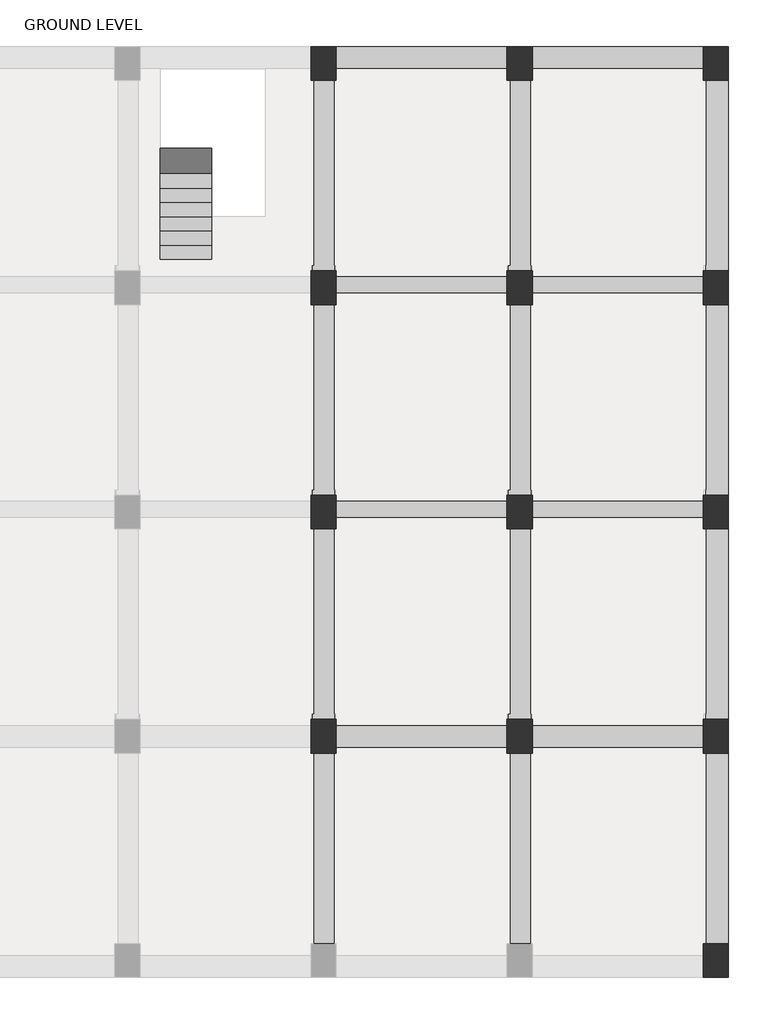
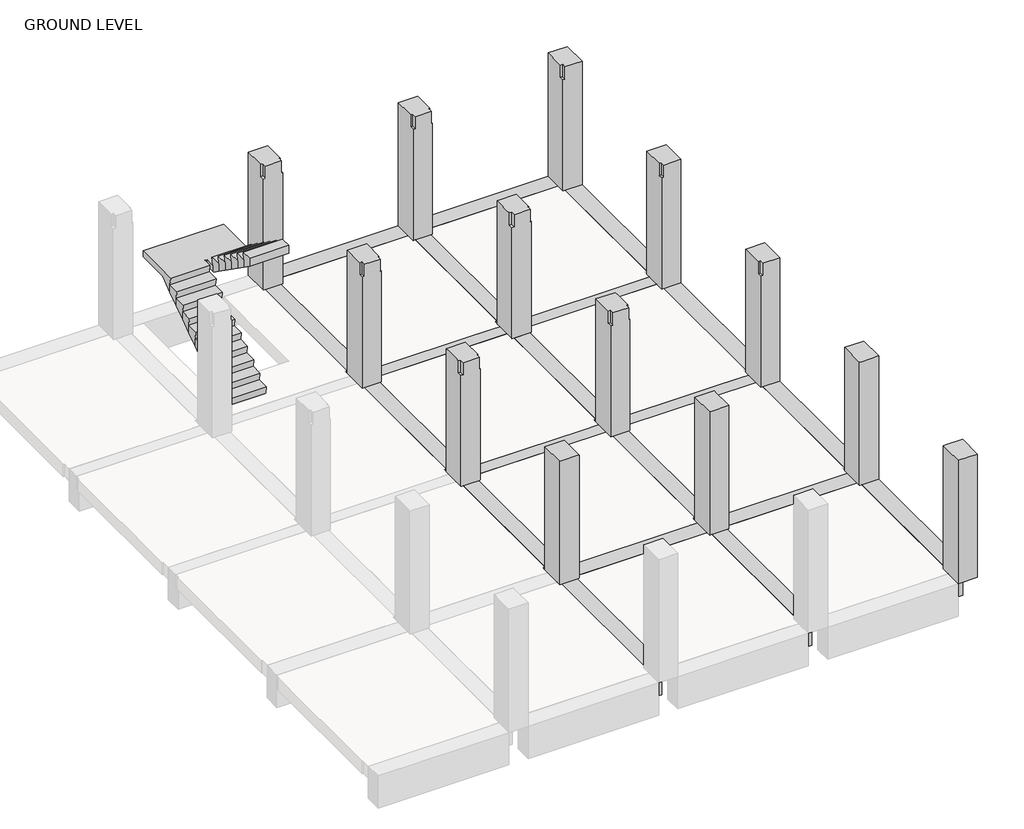
# One storey, part 3 of 3: 20 beams, 13 columns, 1 stair flight.
"""IFC4 building model written with IfcOpenShell, lengths in millimetres."""

from ifc_helpers import new_model, si_unit, origin, place, context, project, spatial, faceted_brep, element, save

model = new_model("IFC4")

# Units and contexts
model_context = context("Model", 3, world=origin())
ifc_project = project(units=[si_unit("LENGTHUNIT", "METRE", prefix="MILLI")], contexts=[model_context])

# Site, building, storey
site = spatial("IfcSite", under=ifc_project)
building = spatial("IfcBuilding", under=site)
storey = spatial("IfcBuildingStorey", under=building, Name="GROUND LEVEL", Elevation=0.0)

# Beams
placement = place(None, origin())
element("IfcBeam", 1, ObjectType="M_Concrete-Rectangular Beam : 400 x 800mm", at=placement, inside=storey, context=model_context, shape_type="Brep", body=[
    faceted_brep([(7955.1115906, 15703.1212443, 0.0), (8355.1115906, 15703.1212443, 0.0), (8355.1115906, 19103.1212443, 0.0), (7955.1115906, 19103.1212443, 0.0), (7955.1115906, 15803.1212443, 0.0), (7955.1115906, 15703.1212443, -800.0), (7955.1115906, 19103.1212443, -800.0), (8355.1115906, 15703.1212443, -800.0), (8355.1115906, 19103.1212443, -800.0)], [[[0, 1, 2, 3, 4]], [[5, 0, 4, 3, 6]], [[7, 5, 6, 8]], [[1, 7, 8, 2]], [[2, 8, 6, 3]], [[1, 0, 5, 7]]]),
])
element("IfcBeam", 2, ObjectType="M_Concrete-Rectangular Beam : 400 x 800mm", at=placement, inside=storey, context=model_context, shape_type="Brep", body=[
    faceted_brep([(7955.1115906, 11703.1212443, 0.0), (8355.1115906, 11703.1212443, 0.0), (8355.1115906, 15103.1212443, 0.0), (7955.1115906, 15103.1212443, 0.0), (7955.1115906, 11803.1212443, 0.0), (7955.1115906, 11703.1212443, -800.0), (7955.1115906, 15103.1212443, -800.0), (8355.1115906, 11703.1212443, -800.0), (8355.1115906, 15103.1212443, -800.0)], [[[0, 1, 2, 3, 4]], [[5, 0, 4, 3, 6]], [[7, 5, 6, 8]], [[1, 7, 8, 2]], [[2, 8, 6, 3]], [[1, 0, 5, 7]]]),
])
element("IfcBeam", 3, ObjectType="M_Concrete-Rectangular Beam : 400 x 800mm", at=placement, inside=storey, context=model_context, shape_type="Brep", body=[
    faceted_brep([(7955.1115906, 7703.1212443, 0.0), (8355.1115906, 7703.1212443, 0.0), (8355.1115906, 11103.1212443, 0.0), (7955.1115906, 11103.1212443, 0.0), (7955.1115906, 7803.1212443, 0.0), (7955.1115906, 7703.1212443, -800.0), (7955.1115906, 11103.1212443, -800.0), (8355.1115906, 7703.1212443, -800.0), (8355.1115906, 11103.1212443, -800.0)], [[[0, 1, 2, 3, 4]], [[5, 0, 4, 3, 6]], [[7, 5, 6, 8]], [[1, 7, 8, 2]], [[1, 0, 5, 7]], [[3, 2, 8, 6]]]),
])
element("IfcBeam", 4, ObjectType="M_Concrete-Rectangular Beam : 400 x 800mm", at=placement, inside=storey, context=model_context, shape_type="Brep", body=[
    faceted_brep([(8355.1115906, 7103.1212443, 0.0), (7955.1115906, 7103.1212443, 0.0), (7955.1115906, 3703.1212443, 0.0), (8355.1115906, 3703.1212443, 0.0), (7955.1115906, 7103.1212443, -300.0), (7955.1115906, 7103.1212443, -800.0), (7955.1115906, 3703.1212443, -800.0), (7955.1115906, 3703.1212443, -300.0), (8355.1115906, 7103.1212443, -800.0), (8355.1115906, 3703.1212443, -800.0)], [[[0, 1, 2, 3]], [[1, 4, 5, 6, 7, 2]], [[5, 8, 9, 6]], [[8, 0, 3, 9]], [[0, 8, 5, 4, 1]], [[3, 2, 7, 6, 9]]]),
])
element("IfcBeam", 5, ObjectType="M_Concrete-Rectangular Beam : 400 x 800mm", at=placement, inside=storey, context=model_context, shape_type="Brep", body=[
    faceted_brep([(1355.1115906, 19703.1212443, 0.0), (1355.1115906, 19303.1212443, 0.0), (4405.1115906, 19303.1212443, 0.0), (4405.1115906, 19703.1212443, 0.0), (1355.1115906, 19303.1212443, -300.0), (1355.1115906, 19303.1212443, -800.0), (4405.1115906, 19303.1212443, -800.0), (4405.1115906, 19303.1212443, -300.0), (1355.1115906, 19703.1212443, -800.0), (4405.1115906, 19703.1212443, -800.0)], [[[0, 1, 2, 3]], [[1, 4, 5, 6, 7, 2]], [[5, 8, 9, 6]], [[8, 0, 3, 9]], [[1, 0, 8, 5, 4]], [[3, 2, 7, 6, 9]]]),
])
element("IfcBeam", 6, ObjectType="M_Concrete-Rectangular Beam : 400 x 800mm", at=placement, inside=storey, context=model_context, shape_type="Brep", body=[
    faceted_brep([(4855.1115906, 19703.1212443, 0.0), (4855.1115906, 19303.1212443, 0.0), (7905.1115906, 19303.1212443, 0.0), (7905.1115906, 19703.1212443, 0.0), (4855.1115906, 19303.1212443, -300.0), (4855.1115906, 19303.1212443, -800.0), (7905.1115906, 19303.1212443, -800.0), (7905.1115906, 19303.1212443, -300.0), (4855.1115906, 19703.1212443, -800.0), (7905.1115906, 19703.1212443, -800.0)], [[[0, 1, 2, 3]], [[1, 4, 5, 6, 7, 2]], [[5, 8, 9, 6]], [[8, 0, 3, 9]], [[1, 0, 8, 5, 4]], [[3, 2, 7, 6, 9]]]),
])
element("IfcBeam", 7, ObjectType="M_Concrete-Rectangular Beam : 400 x 800mm", at=placement, inside=storey, context=model_context, shape_type="Brep", body=[
    faceted_brep([(1330.1115906, 15703.1212443, 0.0), (1330.1115906, 15803.1212443, 0.0), (1330.1115906, 19103.1212443, 0.0), (955.1115906, 19103.1212443, 0.0), (955.1115906, 15803.1212443, 0.0), (930.1115906, 15803.1212443, 0.0), (930.1115906, 15703.1212443, 0.0), (930.1115906, 19103.1212443, -800.0), (930.1115906, 15703.1212443, -800.0), (930.1115906, 15803.1212443, -300.0), (930.1115906, 19103.1212443, -300.0), (1330.1115906, 19103.1212443, -800.0), (1330.1115906, 15703.1212443, -800.0), (955.1115906, 19103.1212443, -300.0), (955.1115906, 15803.1212443, -300.0)], [[[0, 1, 2, 3, 4, 5, 6]], [[7, 8, 6, 5, 9, 10]], [[7, 11, 12, 8]], [[11, 2, 1, 0, 12]], [[2, 11, 7, 10, 13, 3]], [[0, 6, 8, 12]], [[9, 14, 13, 10]], [[14, 4, 3, 13]], [[4, 14, 9, 5]]]),
])
element("IfcBeam", 8, ObjectType="M_Concrete-Rectangular Beam : 400 x 800mm", at=placement, inside=storey, context=model_context, shape_type="Brep", body=[
    faceted_brep([(1330.1115906, 11703.1212443, 0.0), (1330.1115906, 11803.1212443, 0.0), (1330.1115906, 15103.1212443, 0.0), (955.1115906, 15103.1212443, 0.0), (955.1115906, 11803.1212443, 0.0), (930.1115906, 11803.1212443, 0.0), (930.1115906, 11703.1212443, 0.0), (930.1115906, 15103.1212443, -800.0), (930.1115906, 11703.1212443, -800.0), (930.1115906, 11803.1212443, -300.0), (930.1115906, 15103.1212443, -300.0), (1330.1115906, 15103.1212443, -800.0), (1330.1115906, 11703.1212443, -800.0), (955.1115906, 15103.1212443, -300.0), (955.1115906, 11803.1212443, -300.0)], [[[0, 1, 2, 3, 4, 5, 6]], [[7, 8, 6, 5, 9, 10]], [[8, 7, 11, 12]], [[2, 1, 0, 12, 11]], [[2, 11, 7, 10, 13, 3]], [[0, 6, 8, 12]], [[9, 14, 13, 10]], [[14, 4, 3, 13]], [[4, 14, 9, 5]]]),
])
element("IfcBeam", 9, ObjectType="M_Concrete-Rectangular Beam : 400 x 800mm", at=placement, inside=storey, context=model_context, shape_type="Brep", body=[
    faceted_brep([(1330.1115906, 7703.1212443, 0.0), (1330.1115906, 7803.1212443, 0.0), (1330.1115906, 11103.1212443, 0.0), (955.1115906, 11103.1212443, 0.0), (955.1115906, 7803.1212443, 0.0), (930.1115906, 7803.1212443, 0.0), (930.1115906, 7703.1212443, 0.0), (930.1115906, 11103.1212443, -800.0), (930.1115906, 7703.1212443, -800.0), (930.1115906, 7803.1212443, -300.0), (930.1115906, 11103.1212443, -300.0), (1330.1115906, 11103.1212443, -800.0), (1330.1115906, 7703.1212443, -800.0), (955.1115906, 11103.1212443, -300.0), (955.1115906, 7803.1212443, -300.0)], [[[0, 1, 2, 3, 4, 5, 6]], [[7, 8, 6, 5, 9, 10]], [[7, 11, 12, 8]], [[11, 2, 1, 0, 12]], [[2, 11, 7, 10, 13, 3]], [[0, 6, 8, 12]], [[9, 14, 13, 10]], [[14, 4, 3, 13]], [[4, 14, 9, 5]]]),
])
element("IfcBeam", 10, ObjectType="M_Concrete-Rectangular Beam : 400 x 800mm", at=placement, inside=storey, context=model_context, shape_type="Brep", body=[
    faceted_brep([(1330.1115906, 3703.1212443, 0.0), (1330.1115906, 7103.1212443, 0.0), (955.1115906, 7103.1212443, 0.0), (955.1115906, 3703.1212443, 0.0), (930.1115906, 7103.1212443, -800.0), (930.1115906, 3703.1212443, -800.0), (930.1115906, 3703.1212443, -300.0), (930.1115906, 7103.1212443, -300.0), (1330.1115906, 7103.1212443, -800.0), (1330.1115906, 3703.1212443, -800.0), (1330.1115906, 7103.1212443, -300.0), (1330.1115906, 3703.1212443, -300.0), (955.1115906, 7103.1212443, -300.0), (955.1115906, 3703.1212443, -300.0)], [[[0, 1, 2, 3]], [[4, 5, 6, 7]], [[4, 8, 9, 5]], [[8, 10, 1, 0, 11, 9]], [[8, 4, 7, 12, 2, 1, 10]], [[5, 9, 11, 0, 3, 13, 6]], [[13, 12, 7, 6]], [[12, 13, 3, 2]]]),
])
element("IfcBeam", 11, ObjectType="M_Concrete-Rectangular Beam : 400 x 800mm", at=placement, inside=storey, context=model_context, shape_type="Brep", body=[
    faceted_brep([(4830.1115906, 15703.1212443, 0.0), (4830.1115906, 15803.1212443, 0.0), (4830.1115906, 19103.1212443, 0.0), (4455.1115906, 19103.1212443, 0.0), (4455.1115906, 15803.1212443, 0.0), (4430.1115906, 15803.1212443, 0.0), (4430.1115906, 15703.1212443, 0.0), (4430.1115906, 19103.1212443, -800.0), (4430.1115906, 15703.1212443, -800.0), (4430.1115906, 15803.1212443, -300.0), (4430.1115906, 19103.1212443, -300.0), (4830.1115906, 19103.1212443, -800.0), (4830.1115906, 15703.1212443, -800.0), (4455.1115906, 19103.1212443, -300.0), (4455.1115906, 15803.1212443, -300.0)], [[[0, 1, 2, 3, 4, 5, 6]], [[7, 8, 6, 5, 9, 10]], [[8, 7, 11, 12]], [[2, 1, 0, 12, 11]], [[2, 11, 7, 10, 13, 3]], [[0, 6, 8, 12]], [[9, 14, 13, 10]], [[14, 4, 3, 13]], [[4, 14, 9, 5]]]),
])
element("IfcBeam", 12, ObjectType="M_Concrete-Rectangular Beam : 400 x 800mm", at=placement, inside=storey, context=model_context, shape_type="Brep", body=[
    faceted_brep([(4830.1115906, 11703.1212443, 0.0), (4830.1115906, 11803.1212443, 0.0), (4830.1115906, 15103.1212443, 0.0), (4455.1115906, 15103.1212443, 0.0), (4455.1115906, 11803.1212443, 0.0), (4430.1115906, 11803.1212443, 0.0), (4430.1115906, 11703.1212443, 0.0), (4430.1115906, 15103.1212443, -800.0), (4430.1115906, 11703.1212443, -800.0), (4430.1115906, 11803.1212443, -300.0), (4430.1115906, 15103.1212443, -300.0), (4830.1115906, 15103.1212443, -800.0), (4830.1115906, 11703.1212443, -800.0), (4455.1115906, 15103.1212443, -300.0), (4455.1115906, 11803.1212443, -300.0)], [[[0, 1, 2, 3, 4, 5, 6]], [[7, 8, 6, 5, 9, 10]], [[7, 11, 12, 8]], [[11, 2, 1, 0, 12]], [[2, 11, 7, 10, 13, 3]], [[0, 6, 8, 12]], [[9, 14, 13, 10]], [[14, 4, 3, 13]], [[4, 14, 9, 5]]]),
])
element("IfcBeam", 13, ObjectType="M_Concrete-Rectangular Beam : 400 x 800mm", at=placement, inside=storey, context=model_context, shape_type="Brep", body=[
    faceted_brep([(4430.1115906, 7703.1212443, 0.0), (4830.1115906, 7703.1212443, 0.0), (4830.1115906, 7803.1212443, 0.0), (4830.1115906, 11103.1212443, 0.0), (4455.1115906, 11103.1212443, 0.0), (4455.1115906, 7803.1212443, 0.0), (4430.1115906, 7803.1212443, 0.0), (4430.1115906, 7703.1212443, -800.0), (4430.1115906, 7803.1212443, -300.0), (4430.1115906, 11103.1212443, -300.0), (4430.1115906, 11103.1212443, -800.0), (4830.1115906, 7703.1212443, -800.0), (4830.1115906, 11103.1212443, -800.0), (4455.1115906, 11103.1212443, -300.0), (4455.1115906, 7803.1212443, -300.0)], [[[0, 1, 2, 3, 4, 5, 6]], [[7, 0, 6, 8, 9, 10]], [[11, 7, 10, 12]], [[1, 11, 12, 3, 2]], [[1, 0, 7, 11]], [[12, 10, 9, 13, 4, 3]], [[8, 14, 13, 9]], [[14, 5, 4, 13]], [[5, 14, 8, 6]]]),
])
element("IfcBeam", 14, ObjectType="M_Concrete-Rectangular Beam : 400 x 800mm", at=placement, inside=storey, context=model_context, shape_type="Brep", body=[
    faceted_brep([(4830.1115906, 3703.1212443, 0.0), (4830.1115906, 7103.1212443, 0.0), (4455.1115906, 7103.1212443, 0.0), (4455.1115906, 3703.1212443, 0.0), (4430.1115906, 7103.1212443, -800.0), (4430.1115906, 3703.1212443, -800.0), (4430.1115906, 3703.1212443, -300.0), (4430.1115906, 7103.1212443, -300.0), (4830.1115906, 7103.1212443, -800.0), (4830.1115906, 3703.1212443, -800.0), (4830.1115906, 7103.1212443, -300.0), (4830.1115906, 3703.1212443, -300.0), (4455.1115906, 7103.1212443, -300.0), (4455.1115906, 3703.1212443, -300.0)], [[[0, 1, 2, 3]], [[4, 5, 6, 7]], [[4, 8, 9, 5]], [[8, 10, 1, 0, 11, 9]], [[1, 10, 8, 4, 7, 12, 2]], [[5, 9, 11, 0, 3, 13, 6]], [[13, 12, 7, 6]], [[12, 13, 3, 2]]]),
])
element("IfcBeam", 15, ObjectType="M_Concrete-Rectangular Beam : 400 x 800mm", at=placement, inside=storey, context=model_context, shape_type="Brep", body=[
    faceted_brep([(4405.1115906, 15603.1212443, 0.0), (1355.1115906, 15603.1212443, 0.0), (1355.1115906, 15303.1212443, 0.0), (4405.1115906, 15303.1212443, 0.0), (1355.1115906, 15203.1212443, -800.0), (4405.1115906, 15203.1212443, -800.0), (4405.1115906, 15203.1212443, -300.0), (1355.1115906, 15203.1212443, -300.0), (1355.1115906, 15603.1212443, -800.0), (4405.1115906, 15603.1212443, -800.0), (1355.1115906, 15603.1212443, -300.0), (4405.1115906, 15603.1212443, -300.0), (1355.1115906, 15303.1212443, -300.0), (4405.1115906, 15303.1212443, -300.0)], [[[0, 1, 2, 3]], [[4, 5, 6, 7]], [[4, 8, 9, 5]], [[8, 10, 1, 0, 11, 9]], [[8, 4, 7, 12, 2, 1, 10]], [[5, 9, 11, 0, 3, 13, 6]], [[13, 12, 7, 6]], [[12, 13, 3, 2]]]),
])
element("IfcBeam", 16, ObjectType="M_Concrete-Rectangular Beam : 400 x 800mm", at=placement, inside=storey, context=model_context, shape_type="Brep", body=[
    faceted_brep([(7905.1115906, 15603.1212443, 0.0), (4855.1115906, 15603.1212443, 0.0), (4855.1115906, 15303.1212443, 0.0), (7905.1115906, 15303.1212443, 0.0), (4855.1115906, 15203.1212443, -800.0), (7905.1115906, 15203.1212443, -800.0), (7905.1115906, 15203.1212443, -300.0), (4855.1115906, 15203.1212443, -300.0), (4855.1115906, 15603.1212443, -800.0), (7905.1115906, 15603.1212443, -800.0), (4855.1115906, 15603.1212443, -300.0), (7905.1115906, 15603.1212443, -300.0), (4855.1115906, 15303.1212443, -300.0), (7905.1115906, 15303.1212443, -300.0)], [[[0, 1, 2, 3]], [[4, 5, 6, 7]], [[4, 8, 9, 5]], [[8, 10, 1, 0, 11, 9]], [[8, 4, 7, 12, 2, 1, 10]], [[5, 9, 11, 0, 3, 13, 6]], [[13, 12, 7, 6]], [[12, 13, 3, 2]]]),
])
element("IfcBeam", 17, ObjectType="M_Concrete-Rectangular Beam : 400 x 800mm", at=placement, inside=storey, context=model_context, shape_type="Brep", body=[
    faceted_brep([(7905.1115906, 11603.1212443, 0.0), (4855.1115906, 11603.1212443, 0.0), (4855.1115906, 11303.1212443, 0.0), (7905.1115906, 11303.1212443, 0.0), (4855.1115906, 11603.1212443, -800.0), (4855.1115906, 11603.1212443, -300.0), (7905.1115906, 11603.1212443, -300.0), (7905.1115906, 11603.1212443, -800.0), (4855.1115906, 11203.1212443, -800.0), (7905.1115906, 11203.1212443, -800.0), (7905.1115906, 11203.1212443, -300.0), (4855.1115906, 11203.1212443, -300.0), (4855.1115906, 11303.1212443, -300.0), (7905.1115906, 11303.1212443, -300.0)], [[[0, 1, 2, 3]], [[4, 5, 1, 0, 6, 7]], [[8, 4, 7, 9]], [[8, 9, 10, 11]], [[1, 5, 4, 8, 11, 12, 2]], [[7, 6, 0, 3, 13, 10, 9]], [[13, 12, 11, 10]], [[12, 13, 3, 2]]]),
])
element("IfcBeam", 18, ObjectType="M_Concrete-Rectangular Beam : 400 x 800mm", at=placement, inside=storey, context=model_context, shape_type="Brep", body=[
    faceted_brep([(4405.1115906, 11603.1212443, 0.0), (1355.1115906, 11603.1212443, 0.0), (1355.1115906, 11303.1212443, 0.0), (4405.1115906, 11303.1212443, 0.0), (1355.1115906, 11603.1212443, -800.0), (1355.1115906, 11603.1212443, -300.0), (4405.1115906, 11603.1212443, -300.0), (4405.1115906, 11603.1212443, -800.0), (1355.1115906, 11203.1212443, -800.0), (4405.1115906, 11203.1212443, -800.0), (4405.1115906, 11203.1212443, -300.0), (1355.1115906, 11203.1212443, -300.0), (1355.1115906, 11303.1212443, -300.0), (4405.1115906, 11303.1212443, -300.0)], [[[0, 1, 2, 3]], [[4, 5, 1, 0, 6, 7]], [[8, 4, 7, 9]], [[8, 9, 10, 11]], [[1, 5, 4, 8, 11, 12, 2]], [[7, 6, 0, 3, 13, 10, 9]], [[13, 12, 11, 10]], [[12, 13, 3, 2]]]),
])
element("IfcBeam", 19, ObjectType="M_Concrete-Rectangular Beam : 400 x 800mm", at=placement, inside=storey, context=model_context, shape_type="Brep", body=[
    faceted_brep([(1355.1115906, 7603.1212443, 0.0), (1355.1115906, 7203.1212443, 0.0), (4405.1115906, 7203.1212443, 0.0), (4405.1115906, 7603.1212443, 0.0), (1355.1115906, 7203.1212443, -300.0), (1355.1115906, 7203.1212443, -800.0), (4405.1115906, 7203.1212443, -800.0), (4405.1115906, 7203.1212443, -300.0), (1355.1115906, 7603.1212443, -800.0), (4405.1115906, 7603.1212443, -800.0), (1355.1115906, 7603.1212443, -300.0), (4405.1115906, 7603.1212443, -300.0)], [[[0, 1, 2, 3]], [[1, 4, 5, 6, 7, 2]], [[5, 8, 9, 6]], [[8, 10, 0, 3, 11, 9]], [[1, 0, 10, 8, 5, 4]], [[3, 2, 7, 6, 9, 11]]]),
])
element("IfcBeam", 20, ObjectType="M_Concrete-Rectangular Beam : 400 x 800mm", at=placement, inside=storey, context=model_context, shape_type="Brep", body=[
    faceted_brep([(4855.1115906, 7603.1212443, 0.0), (4855.1115906, 7203.1212443, 0.0), (7905.1115906, 7203.1212443, 0.0), (7905.1115906, 7603.1212443, 0.0), (4855.1115906, 7203.1212443, -300.0), (4855.1115906, 7203.1212443, -800.0), (7905.1115906, 7203.1212443, -800.0), (7905.1115906, 7203.1212443, -300.0), (4855.1115906, 7603.1212443, -800.0), (7905.1115906, 7603.1212443, -800.0), (4855.1115906, 7603.1212443, -300.0), (7905.1115906, 7603.1212443, -300.0)], [[[0, 1, 2, 3]], [[1, 4, 5, 6, 7, 2]], [[5, 8, 9, 6]], [[8, 10, 0, 3, 11, 9]], [[1, 0, 10, 8, 5, 4]], [[3, 2, 7, 6, 9, 11]]]),
])

# Columns
element("IfcColumn", 21, ObjectType="M_Concrete-Rectangular-Column : 450 x 600mm", at=placement, inside=storey, context=model_context, shape_type="Brep", body=[
    faceted_brep([(1355.1115906, 19703.1212443, 0.0), (1355.1115906, 19103.1212443, 0.0), (905.1115906, 19103.1212443, 0.0), (905.1115906, 19703.1212443, 0.0), (1355.1115906, 19703.1212443, 3048.0), (1355.1115906, 19303.1212443, 3048.0), (1355.1115906, 19203.1212443, 3048.0), (1355.1115906, 19203.1212443, 2748.0), (1355.1115906, 19103.1212443, 2748.0), (1330.1115906, 19103.1212443, 2748.0), (1330.1115906, 19103.1212443, 3048.0), (955.1115906, 19103.1212443, 3048.0), (955.1115906, 19103.1212443, 2748.0), (905.1115906, 19103.1212443, 2748.0), (905.1115906, 19203.1212443, 2748.0), (905.1115906, 19203.1212443, 3048.0), (905.1115906, 19303.1212443, 3048.0), (905.1115906, 19703.1212443, 3048.0), (955.1115906, 19203.1212443, 3048.0), (1330.1115906, 19203.1212443, 3048.0), (1330.1115906, 19203.1212443, 2748.0), (955.1115906, 19203.1212443, 2748.0)], [[[0, 1, 2, 3]], [[1, 0, 4, 5, 6, 7, 8]], [[2, 1, 8, 9, 10, 11, 12, 13]], [[3, 2, 13, 14, 15, 16, 17]], [[0, 3, 17, 4]], [[4, 17, 16, 15, 18, 11, 10, 19, 6, 5]], [[7, 20, 9, 8]], [[20, 19, 10, 9]], [[20, 7, 6, 19]], [[21, 14, 13, 12]], [[18, 21, 12, 11]], [[14, 21, 18, 15]]]),
])
element("IfcColumn", 22, ObjectType="M_Concrete-Rectangular-Column : 450 x 600mm", at=placement, inside=storey, context=model_context, shape_type="Brep", body=[
    faceted_brep([(4855.1115906, 19703.1212443, 0.0), (4855.1115906, 19103.1212443, 0.0), (4405.1115906, 19103.1212443, 0.0), (4405.1115906, 19703.1212443, 0.0), (4855.1115906, 19703.1212443, 3048.0), (4855.1115906, 19303.1212443, 3048.0), (4855.1115906, 19203.1212443, 3048.0), (4855.1115906, 19203.1212443, 2748.0), (4855.1115906, 19103.1212443, 2748.0), (4830.1115906, 19103.1212443, 2748.0), (4830.1115906, 19103.1212443, 3048.0), (4455.1115906, 19103.1212443, 3048.0), (4455.1115906, 19103.1212443, 2748.0), (4405.1115906, 19103.1212443, 2748.0), (4405.1115906, 19203.1212443, 2748.0), (4405.1115906, 19203.1212443, 3048.0), (4405.1115906, 19303.1212443, 3048.0), (4405.1115906, 19703.1212443, 3048.0), (4455.1115906, 19203.1212443, 3048.0), (4830.1115906, 19203.1212443, 3048.0), (4830.1115906, 19203.1212443, 2748.0), (4455.1115906, 19203.1212443, 2748.0)], [[[0, 1, 2, 3]], [[1, 0, 4, 5, 6, 7, 8]], [[2, 1, 8, 9, 10, 11, 12, 13]], [[3, 2, 13, 14, 15, 16, 17]], [[0, 3, 17, 4]], [[4, 17, 16, 15, 18, 11, 10, 19, 6, 5]], [[7, 20, 9, 8]], [[20, 19, 10, 9]], [[20, 7, 6, 19]], [[21, 14, 13, 12]], [[18, 21, 12, 11]], [[14, 21, 18, 15]]]),
])
element("IfcColumn", 23, ObjectType="M_Concrete-Rectangular-Column : 450 x 600mm", at=placement, inside=storey, context=model_context, shape_type="Brep", body=[
    faceted_brep([(8355.1115906, 19703.1212443, 0.0), (8355.1115906, 19103.1212443, 0.0), (7905.1115906, 19103.1212443, 0.0), (7905.1115906, 19703.1212443, 0.0), (8355.1115906, 19703.1212443, 3048.0), (8355.1115906, 19103.1212443, 3048.0), (7955.1115906, 19103.1212443, 3048.0), (7955.1115906, 19103.1212443, 2748.0), (7905.1115906, 19103.1212443, 2748.0), (7905.1115906, 19203.1212443, 2748.0), (7905.1115906, 19203.1212443, 3048.0), (7905.1115906, 19303.1212443, 3048.0), (7905.1115906, 19703.1212443, 3048.0), (7955.1115906, 19203.1212443, 3048.0), (7955.1115906, 19203.1212443, 2748.0)], [[[0, 1, 2, 3]], [[1, 0, 4, 5]], [[2, 1, 5, 6, 7, 8]], [[3, 2, 8, 9, 10, 11, 12]], [[0, 3, 12, 4]], [[5, 4, 12, 11, 10, 13, 6]], [[14, 9, 8, 7]], [[13, 14, 7, 6]], [[9, 14, 13, 10]]]),
])
element("IfcColumn", 24, ObjectType="M_Concrete-Rectangular-Column : 450 x 600mm", at=placement, inside=storey, context=model_context, shape_type="Brep", body=[
    faceted_brep([(1355.1115906, 15703.1212443, 0.0), (1355.1115906, 15103.1212443, 0.0), (905.1115906, 15103.1212443, 0.0), (905.1115906, 15703.1212443, 0.0), (1355.1115906, 15703.1212443, 2748.0), (1355.1115906, 15703.1212443, 3048.0), (1355.1115906, 15603.1212443, 3048.0), (1355.1115906, 15303.1212443, 3048.0), (1355.1115906, 15203.1212443, 3048.0), (1355.1115906, 15203.1212443, 2748.0), (1355.1115906, 15103.1212443, 2748.0), (1330.1115906, 15103.1212443, 2748.0), (1330.1115906, 15103.1212443, 3048.0), (955.1115906, 15103.1212443, 3048.0), (955.1115906, 15103.1212443, 2748.0), (905.1115906, 15103.1212443, 2748.0), (905.1115906, 15203.1212443, 2748.0), (905.1115906, 15203.1212443, 3048.0), (905.1115906, 15303.1212443, 3048.0), (905.1115906, 15603.1212443, 3048.0), (905.1115906, 15703.1212443, 3048.0), (905.1115906, 15703.1212443, 2748.0), (955.1115906, 15203.1212443, 3048.0), (1330.1115906, 15203.1212443, 3048.0), (1330.1115906, 15203.1212443, 2748.0), (955.1115906, 15203.1212443, 2748.0)], [[[0, 1, 2, 3]], [[1, 0, 4, 5, 6, 7, 8, 9, 10]], [[2, 1, 10, 11, 12, 13, 14, 15]], [[3, 2, 15, 16, 17, 18, 19, 20, 21]], [[0, 3, 21, 20, 5, 4]], [[5, 20, 19, 18, 17, 22, 13, 12, 23, 8, 7, 6]], [[9, 24, 11, 10]], [[24, 23, 12, 11]], [[24, 9, 8, 23]], [[25, 16, 15, 14]], [[22, 25, 14, 13]], [[16, 25, 22, 17]]]),
])
element("IfcColumn", 25, ObjectType="M_Concrete-Rectangular-Column : 450 x 600mm", at=placement, inside=storey, context=model_context, shape_type="Brep", body=[
    faceted_brep([(4855.1115906, 15703.1212443, 0.0), (4855.1115906, 15103.1212443, 0.0), (4405.1115906, 15103.1212443, 0.0), (4405.1115906, 15703.1212443, 0.0), (4855.1115906, 15703.1212443, 2748.0), (4855.1115906, 15703.1212443, 3048.0), (4855.1115906, 15603.1212443, 3048.0), (4855.1115906, 15303.1212443, 3048.0), (4855.1115906, 15203.1212443, 3048.0), (4855.1115906, 15203.1212443, 2748.0), (4855.1115906, 15103.1212443, 2748.0), (4830.1115906, 15103.1212443, 2748.0), (4830.1115906, 15103.1212443, 3048.0), (4455.1115906, 15103.1212443, 3048.0), (4455.1115906, 15103.1212443, 2748.0), (4405.1115906, 15103.1212443, 2748.0), (4405.1115906, 15203.1212443, 2748.0), (4405.1115906, 15203.1212443, 3048.0), (4405.1115906, 15303.1212443, 3048.0), (4405.1115906, 15603.1212443, 3048.0), (4405.1115906, 15703.1212443, 3048.0), (4405.1115906, 15703.1212443, 2748.0), (4455.1115906, 15203.1212443, 3048.0), (4830.1115906, 15203.1212443, 3048.0), (4830.1115906, 15203.1212443, 2748.0), (4455.1115906, 15203.1212443, 2748.0)], [[[0, 1, 2, 3]], [[1, 0, 4, 5, 6, 7, 8, 9, 10]], [[2, 1, 10, 11, 12, 13, 14, 15]], [[3, 2, 15, 16, 17, 18, 19, 20, 21]], [[0, 3, 21, 20, 5, 4]], [[5, 20, 19, 18, 17, 22, 13, 12, 23, 8, 7, 6]], [[9, 24, 11, 10]], [[24, 23, 12, 11]], [[24, 9, 8, 23]], [[25, 16, 15, 14]], [[22, 25, 14, 13]], [[16, 25, 22, 17]]]),
])
element("IfcColumn", 26, ObjectType="M_Concrete-Rectangular-Column : 450 x 600mm", at=placement, inside=storey, context=model_context, shape_type="Brep", body=[
    faceted_brep([(8355.1115906, 15703.1212443, 0.0), (8355.1115906, 15103.1212443, 0.0), (7905.1115906, 15103.1212443, 0.0), (7905.1115906, 15703.1212443, 0.0), (8355.1115906, 15703.1212443, 3048.0), (8355.1115906, 15103.1212443, 3048.0), (7955.1115906, 15103.1212443, 3048.0), (7955.1115906, 15103.1212443, 2748.0), (7905.1115906, 15103.1212443, 2748.0), (7905.1115906, 15203.1212443, 2748.0), (7905.1115906, 15203.1212443, 3048.0), (7905.1115906, 15303.1212443, 3048.0), (7905.1115906, 15603.1212443, 3048.0), (7905.1115906, 15703.1212443, 3048.0), (7905.1115906, 15703.1212443, 2748.0), (7955.1115906, 15203.1212443, 3048.0), (7955.1115906, 15203.1212443, 2748.0)], [[[0, 1, 2, 3]], [[1, 0, 4, 5]], [[2, 1, 5, 6, 7, 8]], [[3, 2, 8, 9, 10, 11, 12, 13, 14]], [[0, 3, 14, 13, 4]], [[5, 4, 13, 12, 11, 10, 15, 6]], [[16, 9, 8, 7]], [[15, 16, 7, 6]], [[9, 16, 15, 10]]]),
])
element("IfcColumn", 27, ObjectType="M_Concrete-Rectangular-Column : 450 x 600mm", at=placement, inside=storey, context=model_context, shape_type="Brep", body=[
    faceted_brep([(1355.1115906, 11703.1212443, 0.0), (1355.1115906, 11103.1212443, 0.0), (905.1115906, 11103.1212443, 0.0), (905.1115906, 11703.1212443, 0.0), (1355.1115906, 11703.1212443, 2748.0), (1355.1115906, 11703.1212443, 3048.0), (1355.1115906, 11603.1212443, 3048.0), (1355.1115906, 11303.1212443, 3048.0), (1355.1115906, 11203.1212443, 3048.0), (1355.1115906, 11203.1212443, 2748.0), (1355.1115906, 11103.1212443, 2748.0), (1330.1115906, 11103.1212443, 2748.0), (1330.1115906, 11103.1212443, 3048.0), (955.1115906, 11103.1212443, 3048.0), (955.1115906, 11103.1212443, 2748.0), (905.1115906, 11103.1212443, 2748.0), (905.1115906, 11203.1212443, 2748.0), (905.1115906, 11203.1212443, 3048.0), (905.1115906, 11303.1212443, 3048.0), (905.1115906, 11603.1212443, 3048.0), (905.1115906, 11703.1212443, 3048.0), (905.1115906, 11703.1212443, 2748.0), (955.1115906, 11203.1212443, 3048.0), (1330.1115906, 11203.1212443, 3048.0), (1330.1115906, 11203.1212443, 2748.0), (955.1115906, 11203.1212443, 2748.0)], [[[0, 1, 2, 3]], [[1, 0, 4, 5, 6, 7, 8, 9, 10]], [[2, 1, 10, 11, 12, 13, 14, 15]], [[3, 2, 15, 16, 17, 18, 19, 20, 21]], [[0, 3, 21, 20, 5, 4]], [[5, 20, 19, 18, 17, 22, 13, 12, 23, 8, 7, 6]], [[9, 24, 11, 10]], [[24, 23, 12, 11]], [[24, 9, 8, 23]], [[25, 16, 15, 14]], [[22, 25, 14, 13]], [[16, 25, 22, 17]]]),
])
element("IfcColumn", 28, ObjectType="M_Concrete-Rectangular-Column : 450 x 600mm", at=placement, inside=storey, context=model_context, shape_type="Brep", body=[
    faceted_brep([(4855.1115906, 11703.1212443, 0.0), (4855.1115906, 11103.1212443, 0.0), (4405.1115906, 11103.1212443, 0.0), (4405.1115906, 11703.1212443, 0.0), (4855.1115906, 11703.1212443, 2748.0), (4855.1115906, 11703.1212443, 3048.0), (4855.1115906, 11603.1212443, 3048.0), (4855.1115906, 11303.1212443, 3048.0), (4855.1115906, 11203.1212443, 3048.0), (4855.1115906, 11203.1212443, 2748.0), (4855.1115906, 11103.1212443, 2748.0), (4830.1115906, 11103.1212443, 2748.0), (4830.1115906, 11103.1212443, 3048.0), (4455.1115906, 11103.1212443, 3048.0), (4455.1115906, 11103.1212443, 2748.0), (4405.1115906, 11103.1212443, 2748.0), (4405.1115906, 11203.1212443, 2748.0), (4405.1115906, 11203.1212443, 3048.0), (4405.1115906, 11303.1212443, 3048.0), (4405.1115906, 11603.1212443, 3048.0), (4405.1115906, 11703.1212443, 3048.0), (4405.1115906, 11703.1212443, 2748.0), (4455.1115906, 11203.1212443, 3048.0), (4830.1115906, 11203.1212443, 3048.0), (4830.1115906, 11203.1212443, 2748.0), (4455.1115906, 11203.1212443, 2748.0)], [[[0, 1, 2, 3]], [[1, 0, 4, 5, 6, 7, 8, 9, 10]], [[2, 1, 10, 11, 12, 13, 14, 15]], [[3, 2, 15, 16, 17, 18, 19, 20, 21]], [[0, 3, 21, 20, 5, 4]], [[5, 20, 19, 18, 17, 22, 13, 12, 23, 8, 7, 6]], [[9, 24, 11, 10]], [[24, 23, 12, 11]], [[24, 9, 8, 23]], [[25, 16, 15, 14]], [[22, 25, 14, 13]], [[16, 25, 22, 17]]]),
])
element("IfcColumn", 29, ObjectType="M_Concrete-Rectangular-Column : 450 x 600mm", at=placement, inside=storey, context=model_context, shape_type="Brep", body=[
    faceted_brep([(8355.1115906, 11703.1212443, 0.0), (8355.1115906, 11103.1212443, 0.0), (7905.1115906, 11103.1212443, 0.0), (7905.1115906, 11703.1212443, 0.0), (8355.1115906, 11703.1212443, 3048.0), (8355.1115906, 11103.1212443, 3048.0), (7955.1115906, 11103.1212443, 3048.0), (7955.1115906, 11103.1212443, 2748.0), (7905.1115906, 11103.1212443, 2748.0), (7905.1115906, 11203.1212443, 2748.0), (7905.1115906, 11203.1212443, 3048.0), (7905.1115906, 11303.1212443, 3048.0), (7905.1115906, 11603.1212443, 3048.0), (7905.1115906, 11703.1212443, 3048.0), (7905.1115906, 11703.1212443, 2748.0), (7955.1115906, 11203.1212443, 3048.0), (7955.1115906, 11203.1212443, 2748.0)], [[[0, 1, 2, 3]], [[1, 0, 4, 5]], [[2, 1, 5, 6, 7, 8]], [[3, 2, 8, 9, 10, 11, 12, 13, 14]], [[0, 3, 14, 13, 4]], [[5, 4, 13, 12, 11, 10, 15, 6]], [[16, 9, 8, 7]], [[15, 16, 7, 6]], [[9, 16, 15, 10]]]),
])
element("IfcColumn", 30, ObjectType="M_Concrete-Rectangular-Column : 450 x 600mm", at=placement, inside=storey, context=model_context, shape_type="Brep", body=[
    faceted_brep([(1355.1115906, 7703.1212443, 0.0), (1355.1115906, 7103.1212443, 0.0), (905.1115906, 7103.1212443, 0.0), (905.1115906, 7703.1212443, 0.0), (1355.1115906, 7703.1212443, 2748.0), (1355.1115906, 7703.1212443, 3048.0), (1355.1115906, 7603.1212443, 3048.0), (1355.1115906, 7203.1212443, 3048.0), (1355.1115906, 7103.1212443, 3048.0), (1355.1115906, 7103.1212443, 2748.0), (1330.1115906, 7103.1212443, 3048.0), (955.1115906, 7103.1212443, 3048.0), (905.1115906, 7103.1212443, 3048.0), (905.1115906, 7103.1212443, 2748.0), (905.1115906, 7203.1212443, 3048.0), (905.1115906, 7603.1212443, 3048.0), (905.1115906, 7703.1212443, 3048.0), (905.1115906, 7703.1212443, 2748.0)], [[[0, 1, 2, 3]], [[1, 0, 4, 5, 6, 7, 8, 9]], [[2, 1, 9, 8, 10, 11, 12, 13]], [[3, 2, 13, 12, 14, 15, 16, 17]], [[0, 3, 17, 16, 5, 4]], [[5, 16, 15, 14, 12, 11, 10, 8, 7, 6]]]),
])
element("IfcColumn", 31, ObjectType="M_Concrete-Rectangular-Column : 450 x 600mm", at=placement, inside=storey, context=model_context, shape_type="Brep", body=[
    faceted_brep([(4855.1115906, 7703.1212443, 0.0), (4855.1115906, 7103.1212443, 0.0), (4405.1115906, 7103.1212443, 0.0), (4405.1115906, 7703.1212443, 0.0), (4855.1115906, 7703.1212443, 2748.0), (4855.1115906, 7703.1212443, 3048.0), (4855.1115906, 7603.1212443, 3048.0), (4855.1115906, 7203.1212443, 3048.0), (4855.1115906, 7103.1212443, 3048.0), (4855.1115906, 7103.1212443, 2748.0), (4830.1115906, 7103.1212443, 3048.0), (4455.1115906, 7103.1212443, 3048.0), (4405.1115906, 7103.1212443, 3048.0), (4405.1115906, 7103.1212443, 2748.0), (4405.1115906, 7203.1212443, 3048.0), (4405.1115906, 7603.1212443, 3048.0), (4405.1115906, 7703.1212443, 3048.0), (4405.1115906, 7703.1212443, 2748.0)], [[[0, 1, 2, 3]], [[1, 0, 4, 5, 6, 7, 8, 9]], [[2, 1, 9, 8, 10, 11, 12, 13]], [[3, 2, 13, 12, 14, 15, 16, 17]], [[0, 3, 17, 16, 5, 4]], [[5, 16, 15, 14, 12, 11, 10, 8, 7, 6]]]),
])
element("IfcColumn", 32, ObjectType="M_Concrete-Rectangular-Column : 450 x 600mm", at=placement, inside=storey, context=model_context, shape_type="Brep", body=[
    faceted_brep([(8355.1115906, 7703.1212443, 0.0), (8355.1115906, 7103.1212443, 0.0), (7905.1115906, 7103.1212443, 0.0), (7905.1115906, 7703.1212443, 0.0), (8355.1115906, 7703.1212443, 3048.0), (8355.1115906, 7103.1212443, 3048.0), (7955.1115906, 7103.1212443, 3048.0), (7905.1115906, 7103.1212443, 3048.0), (7905.1115906, 7103.1212443, 2748.0), (7905.1115906, 7203.1212443, 3048.0), (7905.1115906, 7603.1212443, 3048.0), (7905.1115906, 7703.1212443, 3048.0), (7905.1115906, 7703.1212443, 2748.0)], [[[0, 1, 2, 3]], [[1, 0, 4, 5]], [[2, 1, 5, 6, 7, 8]], [[3, 2, 8, 7, 9, 10, 11, 12]], [[0, 3, 12, 11, 4]], [[5, 4, 11, 10, 9, 7, 6]]]),
])
element("IfcColumn", 33, ObjectType="M_Concrete-Rectangular-Column : 450 x 600mm", at=placement, inside=storey, context=model_context, shape_type="Brep", body=[
    faceted_brep([(8355.1115906, 3703.1212443, 0.0), (8355.1115906, 3103.1212443, 0.0), (7905.1115906, 3103.1212443, 0.0), (7905.1115906, 3703.1212443, 0.0), (8355.1115906, 3703.1212443, 3048.0), (8355.1115906, 3103.1212443, 3048.0), (7905.1115906, 3103.1212443, 3048.0), (7905.1115906, 3503.1212443, 3048.0), (7905.1115906, 3703.1212443, 3048.0), (7905.1115906, 3703.1212443, 2748.0), (7955.1115906, 3703.1212443, 3048.0)], [[[0, 1, 2, 3]], [[1, 0, 4, 5]], [[2, 1, 5, 6]], [[3, 2, 6, 7, 8, 9]], [[0, 3, 9, 8, 10, 4]], [[5, 4, 10, 8, 7, 6]]]),
])

# Stair flight
element("IfcStairFlight", 34, ObjectType="25 mm Nosing", at=placement, inside=storey, context=model_context, shape_type="Brep", body=[
    faceted_brep([(-1784.8884094, 15908.7212443, 179.2941176), (-870.4884094, 15908.7212443, 179.2941176), (-870.4884094, 16187.7212443, 179.2941176), (-1784.8884094, 16187.7212443, 179.2941176), (-1784.8884094, 16187.7212443, 0.0), (-1784.8884094, 15933.7212443, 0.0), (-870.4884094, 15933.7212443, 0.0), (-870.4884094, 16187.7212443, 0.0), (-1784.8884094, 16162.7212443, 358.5882353), (-870.4884094, 16162.7212443, 358.5882353), (-870.4884094, 16441.7212443, 358.5882353), (-1784.8884094, 16441.7212443, 358.5882353), (-1784.8884094, 16441.7212443, 174.9824819), (-1784.8884094, 16193.8293949, 0.0), (-870.4884094, 16193.8293949, 0.0), (-870.4884094, 16441.7212443, 174.9824819), (-1784.8884094, 16416.7212443, 537.8823529), (-870.4884094, 16416.7212443, 537.8823529), (-870.4884094, 16695.7212443, 537.8823529), (-1784.8884094, 16695.7212443, 537.8823529), (-1784.8884094, 16695.7212443, 354.2765996), (-870.4884094, 16695.7212443, 354.2765996), (-1784.8884094, 16670.7212443, 717.1764706), (-870.4884094, 16670.7212443, 717.1764706), (-870.4884094, 16949.7212443, 717.1764706), (-1784.8884094, 16949.7212443, 717.1764706), (-1784.8884094, 16949.7212443, 533.5707172), (-870.4884094, 16949.7212443, 533.5707172), (-1784.8884094, 16924.7212443, 896.4705882), (-870.4884094, 16924.7212443, 896.4705882), (-870.4884094, 17203.7212443, 896.4705882), (-1784.8884094, 17203.7212443, 896.4705882), (-1784.8884094, 17203.7212443, 712.8648349), (-870.4884094, 17203.7212443, 712.8648349), (-1784.8884094, 17178.7212443, 1075.7647059), (-870.4884094, 17178.7212443, 1075.7647059), (-870.4884094, 17457.7212443, 1075.7647059), (-1784.8884094, 17457.7212443, 1075.7647059), (-1784.8884094, 17457.7212443, 892.1589525), (-870.4884094, 17457.7212443, 892.1589525), (-1784.8884094, 17432.7212443, 1255.0588235), (-870.4884094, 17432.7212443, 1255.0588235), (-870.4884094, 17711.7212443, 1255.0588235), (-1784.8884094, 17711.7212443, 1255.0588235), (-1784.8884094, 17711.7212443, 1071.4530702), (-870.4884094, 17711.7212443, 1071.4530702), (-1784.8884094, 17686.7212443, 1434.3529412), (-870.4884094, 17686.7212443, 1434.3529412), (-870.4884094, 17965.7212443, 1434.3529412), (-1784.8884094, 17965.7212443, 1434.3529412), (-1784.8884094, 17965.7212443, 1250.7471878), (-870.4884094, 17965.7212443, 1250.7471878), (-1784.8884094, 17940.7212443, 1613.6470588), (-870.4884094, 17940.7212443, 1613.6470588), (-870.4884094, 18219.7212443, 1613.6470588), (-1784.8884094, 18219.7212443, 1613.6470588), (-1784.8884094, 18219.7212443, 1430.0413055), (-870.4884094, 18219.7212443, 1430.0413055), (94.7115906, 18169.7212443, 1792.9411765), (94.7115906, 19303.1212443, 1792.9411765), (-1784.8884094, 19303.1212443, 1792.9411765), (-1784.8884094, 18521.3293949, 1792.9411765), (-1784.8884094, 18194.7212443, 1792.9411765), (-870.4884094, 18194.7212443, 1792.9411765), (-870.4884094, 18388.7212443, 1792.9411765), (-819.6884094, 18388.7212443, 1792.9411765), (-819.6884094, 18169.7212443, 1792.9411765), (94.7115906, 18169.7212443, 1642.9411765), (94.7115906, 19303.1212443, 1642.9411765), (-1784.8884094, 19303.1212443, 1642.9411765), (-1784.8884094, 18521.3293949, 1642.9411765), (-870.4884094, 18521.3293949, 1642.9411765), (-870.4884094, 18388.7212443, 1642.9411765), (-819.6884094, 18388.7212443, 1642.9411765), (-819.6884094, 18169.7212443, 1642.9411765), (94.7115906, 18194.7212443, 1972.2352941), (-819.6884094, 18194.7212443, 1972.2352941), (-819.6884094, 18122.1130937, 1972.2352941), (-819.6884094, 17915.7212443, 1972.2352941), (94.7115906, 17915.7212443, 1972.2352941), (94.7115906, 18122.1130937, 1972.2352941), (94.7115906, 17915.7212443, 1788.6295408), (94.7115906, 18122.1130937, 1642.9411765), (-819.6884094, 18122.1130937, 1642.9411765), (-819.6884094, 17915.7212443, 1788.6295408), (94.7115906, 17940.7212443, 2151.5294118), (-819.6884094, 17940.7212443, 2151.5294118), (-819.6884094, 17661.7212443, 2151.5294118), (94.7115906, 17661.7212443, 2151.5294118), (94.7115906, 17661.7212443, 1967.9236584), (-819.6884094, 17661.7212443, 1967.9236584), (94.7115906, 17686.7212443, 2330.8235294), (-819.6884094, 17686.7212443, 2330.8235294), (-819.6884094, 17407.7212443, 2330.8235294), (94.7115906, 17407.7212443, 2330.8235294), (94.7115906, 17407.7212443, 2147.2177761), (-819.6884094, 17407.7212443, 2147.2177761), (94.7115906, 17432.7212443, 2510.1176471), (-819.6884094, 17432.7212443, 2510.1176471), (-819.6884094, 17153.7212443, 2510.1176471), (94.7115906, 17153.7212443, 2510.1176471), (94.7115906, 17153.7212443, 2326.5118937), (-819.6884094, 17153.7212443, 2326.5118937), (94.7115906, 17178.7212443, 2689.4117647), (-819.6884094, 17178.7212443, 2689.4117647), (-819.6884094, 16899.7212443, 2689.4117647), (94.7115906, 16899.7212443, 2689.4117647), (94.7115906, 16899.7212443, 2505.8060114), (-819.6884094, 16899.7212443, 2505.8060114), (94.7115906, 16924.7212443, 2868.7058824), (-819.6884094, 16924.7212443, 2868.7058824), (-819.6884094, 16670.7212443, 2868.7058824), (94.7115906, 16670.7212443, 2868.7058824), (94.7115906, 16670.7212443, 2667.4530702), (-819.6884094, 16670.7212443, 2667.4530702)], [[[0, 1, 2, 3]], [[0, 3, 4, 5]], [[2, 1, 6, 7]], [[8, 9, 10, 11]], [[4, 3, 8, 11, 12, 13]], [[2, 7, 14, 15, 10, 9]], [[16, 17, 18, 19]], [[16, 19, 20, 12, 11]], [[18, 17, 10, 15, 21]], [[22, 23, 24, 25]], [[22, 25, 26, 20, 19]], [[24, 23, 18, 21, 27]], [[28, 29, 30, 31]], [[28, 31, 32, 26, 25]], [[30, 29, 24, 27, 33]], [[34, 35, 36, 37]], [[34, 37, 38, 32, 31]], [[36, 35, 30, 33, 39]], [[40, 41, 42, 43]], [[40, 43, 44, 38, 37]], [[42, 41, 36, 39, 45]], [[46, 47, 48, 49]], [[46, 49, 50, 44, 43]], [[48, 47, 42, 45, 51]], [[52, 53, 54, 55]], [[52, 55, 56, 50, 49]], [[54, 53, 48, 51, 57]], [[58, 59, 60, 61, 62, 63, 64, 65, 66]], [[59, 58, 67, 68]], [[60, 59, 68, 69]], [[55, 62, 61, 60, 69, 70, 56]], [[64, 63, 54, 57, 71, 72]], [[65, 64, 72, 73]], [[66, 65, 73, 74]], [[75, 76, 77, 78, 79, 80]], [[58, 75, 80, 79, 81, 82, 67]], [[76, 66, 74, 83, 84, 78, 77]], [[85, 86, 87, 88]], [[85, 88, 89, 81, 79]], [[87, 86, 78, 84, 90]], [[91, 92, 93, 94]], [[91, 94, 95, 89, 88]], [[93, 92, 87, 90, 96]], [[97, 98, 99, 100]], [[97, 100, 101, 95, 94]], [[99, 98, 93, 96, 102]], [[103, 104, 105, 106]], [[103, 106, 107, 101, 100]], [[105, 104, 99, 102, 108]], [[1, 0, 5, 6]], [[3, 2, 9, 8]], [[11, 10, 17, 16]], [[19, 18, 23, 22]], [[25, 24, 29, 28]], [[31, 30, 35, 34]], [[37, 36, 41, 40]], [[43, 42, 47, 46]], [[49, 48, 53, 52]], [[55, 54, 63, 62]], [[58, 66, 76, 75]], [[79, 78, 86, 85]], [[88, 87, 92, 91]], [[94, 93, 98, 97]], [[100, 99, 104, 103]], [[109, 110, 111, 112]], [[109, 112, 113, 107, 106]], [[111, 110, 105, 108, 114]], [[112, 111, 114, 113]], [[106, 105, 110, 109]], [[5, 4, 13, 14, 7, 6]], [[70, 71, 57, 51, 45, 39, 33, 27, 21, 15, 14, 13, 12, 20, 26, 32, 38, 44, 50, 56]], [[71, 70, 69, 68, 67, 82, 83, 74, 73, 72]], [[83, 82, 81, 89, 95, 101, 107, 113, 114, 108, 102, 96, 90, 84]]]),
])

save(model, "model.ifc")

# Revit data of these elements
# Type "M_Concrete-Rectangular Beam : 400 x 800mm"
#   Length [instance default] = 5' - 0"
#   b = 1' - 3.74803"
#   h = 2' - 7.49606"
#   Structural Material [instance default] = Concrete, Cast-in-Place gray
#   Assembly Code = ""
# Type "M_Concrete-Rectangular-Column : 450 x 600mm"
#   b = 1' - 5.71654"
#   h = 1' - 11.62205"
#   Structural Material [instance default] = Concrete, Cast-in-Place gray
# Elements 1, 2, 3, 4, 5, 6, 7, 8, 9, 10, 11, 12, 13, 14, 15, 16, 17, 18, 19, 20 (IfcBeam, "M_Concrete-Rectangular Beam : 400 x 800mm")
#   Structural Material = Concrete, Cast-in-Place gray
#   Phase Created = New Construction
#   Materials on its faces: "Concrete, Cast-in-Place gray"
# Elements 21, 22, 23, 24, 25, 26, 27, 28, 29, 30, 31, 32, 33 (IfcColumn, "M_Concrete-Rectangular-Column : 450 x 600mm")
#   Structural Material = Concrete, Cast-in-Place gray
#   Phase Created = New Construction
#   Materials on its faces: "Concrete, Cast-in-Place gray"
# Element 34 (IfcStairFlight, "25 mm Nosing")
#   Phase Created = New Construction
#   Materials on its faces: "Concrete, Cast In Situ"
# Materials
#   "Concrete, Cast-in-Place gray": class "Concrete", colour RGB 192 192 192, transparency 0, Description = "Cast-in-place concrete", Cost = 0
#   "Concrete, Cast In Situ": class "Concrete", colour RGB 192 192 192, transparency 0, Description = "physical material", Cost = 0
